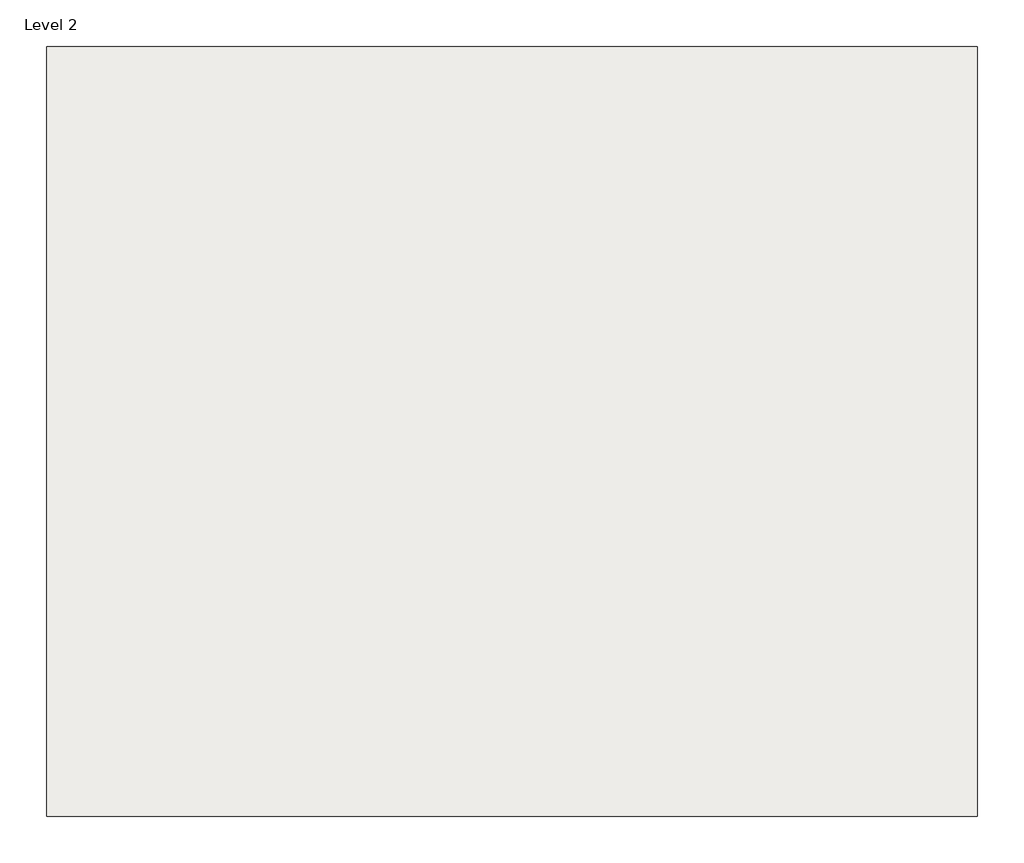
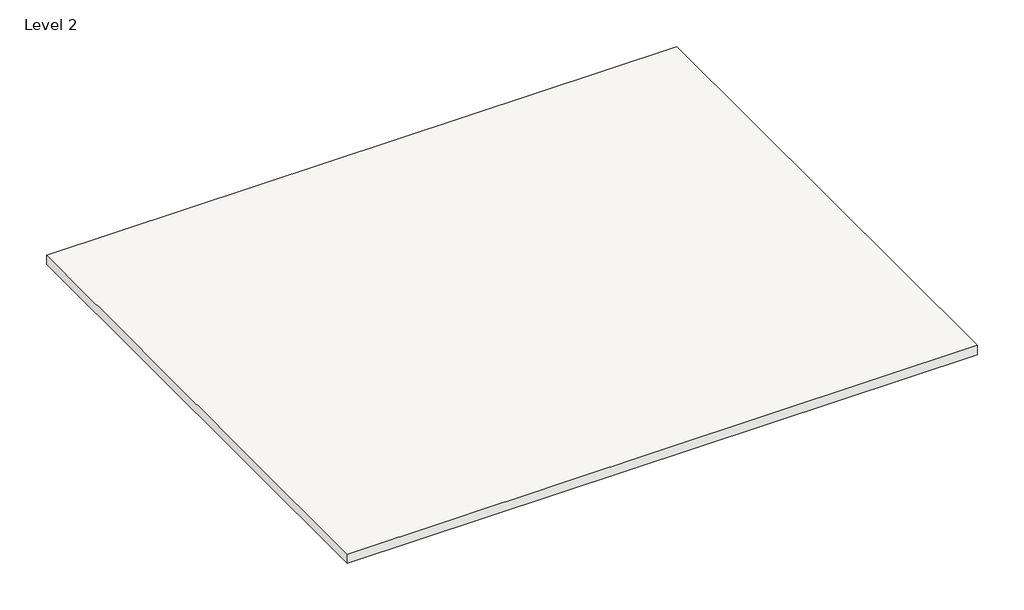
# One storey: 1 roof.
"""IFC4 building model written with IfcOpenShell, lengths in millimetres."""

from ifc_helpers import new_model, si_unit, frame, origin, place, context, project, spatial, polyline, outline, extrude, element, save

model = new_model("IFC4")

# Units and contexts
model_context = context("Model", 3, world=origin())
ifc_project = project(units=[si_unit("LENGTHUNIT", "METRE", prefix="MILLI")], contexts=[model_context])

# Site, building, storey
site = spatial("IfcSite", under=ifc_project)
building = spatial("IfcBuilding", under=site)
storey = spatial("IfcBuildingStorey", under=building, Name="Level 2", Elevation=3048.0)

# Roof
placement = place(None, origin())
element("IfcRoof", 1, ObjectType="Generic - 12\"", at=placement, inside=storey, context=model_context, shape_type="SweptSolid", body=[
    extrude(outline(polyline([(-19307.9871679, 15732.1833409), (681.8128321, 15732.1833409), (681.8128321, -803.2166591), (-19307.9871679, -803.2166591), (-19307.9871679, 15732.1833409)])), frame((0.0, 0.0, 3048.0), z_axis=(0.0, 0.0, 1.0), x_axis=(1.0, 0.0, 0.0)), (0.0, 0.0, 1.0), 304.8),
])

save(model, "model.ifc")

# Revit data of these elements
# Type "Generic - 12\""
#   Assembly Code = "B1020"
#   Layers, outside or top first: 1' - 0" no material (function 1)
# Element 1 (IfcRoof, "Generic - 12\"")
#   built-in parameter 1001705 = 11 (stored number, unit not read)
#   built-in parameter 1001710 = 33615
#   Phase Created = New Construction
#   Materials on its faces: "Default Roof"
# Materials
#   "Default Roof": colour RGB 88 101 114, transparency 0
